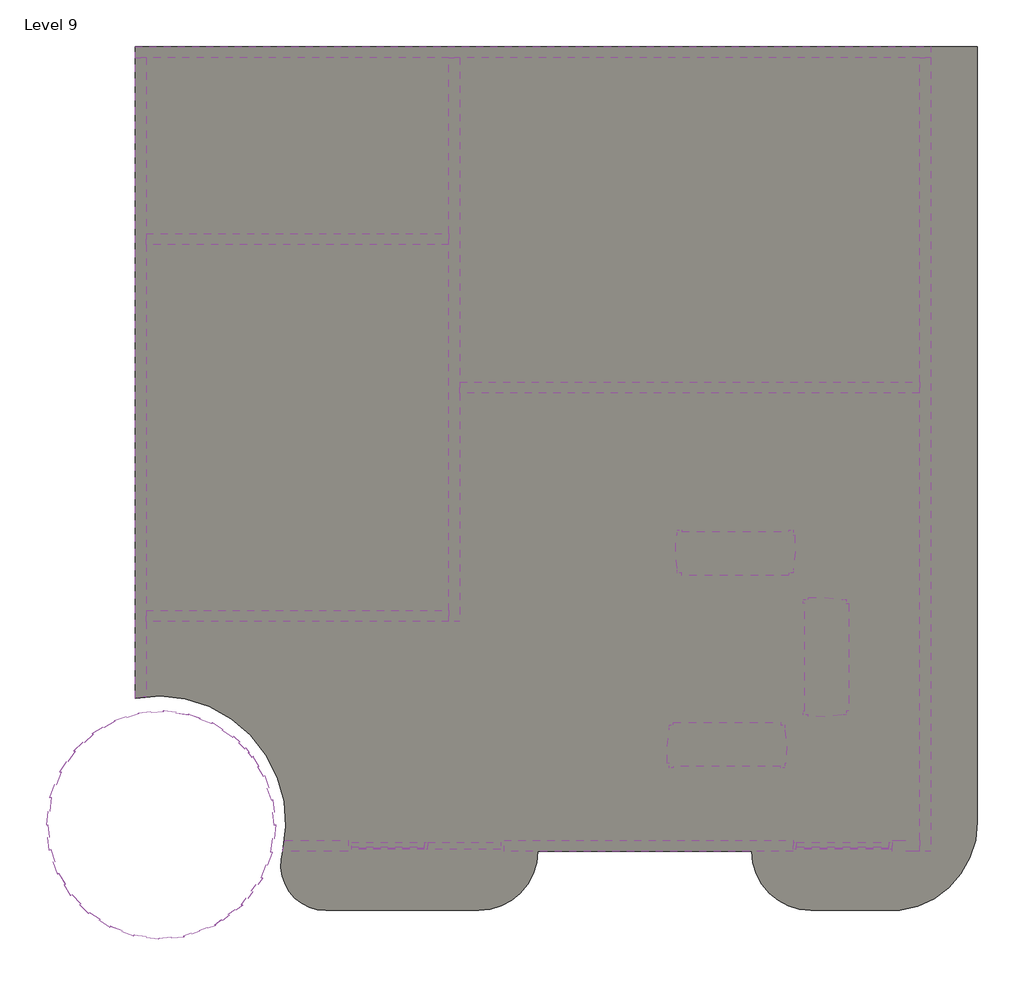
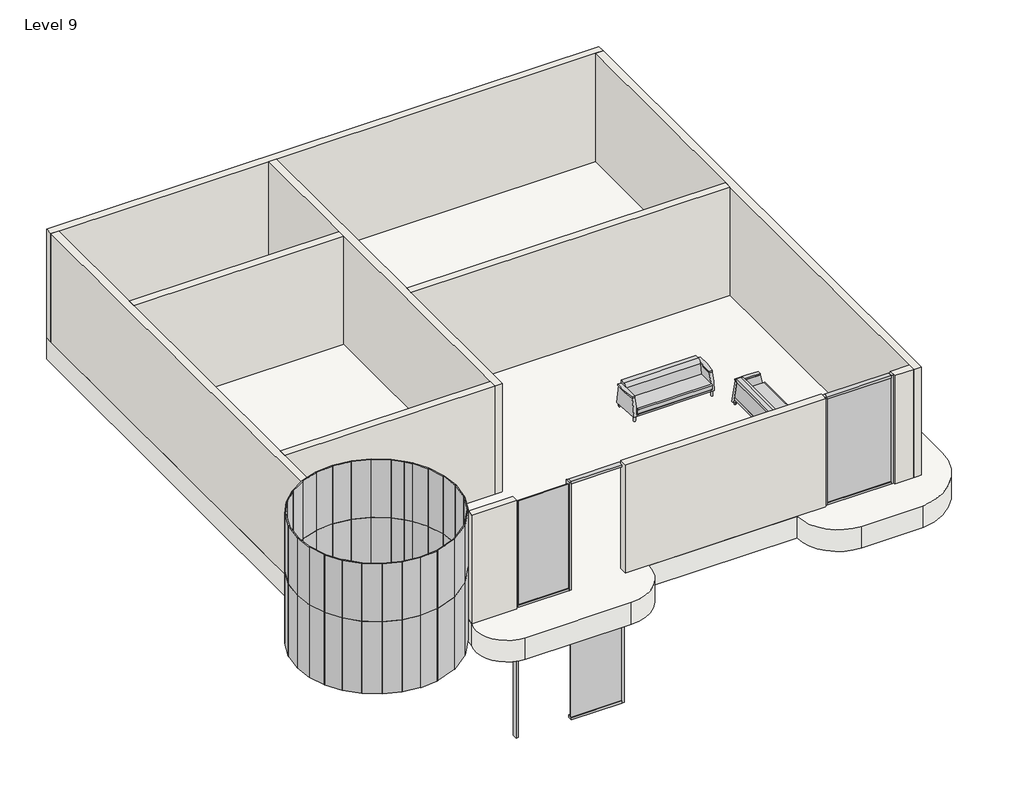
# One storey, incomplete: 59 plates, 11 members, 10 walls, 3 furniture elements, 1 slab.
"""IFC4 building model written with IfcOpenShell, lengths in millimetres."""

from ifc_helpers import new_model, si_unit, point, frame, frame_2d, origin, place, context, project, spatial, polyline, circle_curve, trimmed, segment, composite_curve, outline, extrude, faceted_brep, transform, mapped, element, save
from ifc_brep_helpers import plane_surface, revolved_surface, advanced_brep
from components import furniture_aff9b2fb, member_eaba9652, member_3f395ae9, member_0c868e12, member_7bc42366, system_panel_glazed_f1c144f9, system_panel_glazed_8ed2b2ee, system_panel_glazed_c7815b78, system_panel_glazed_220ba5f3, system_panel_glazed_11fb153e, system_panel_glazed_2f540b85, system_panel_glazed_4848e608, system_panel_glazed_8b35a0ff, system_panel_glazed_87282c25, system_panel_glazed_6d1bb68c, system_panel_glazed_cb3ffd69, system_panel_glazed_404d015f, system_panel_glazed_7b556abe, system_panel_glazed_370bf902

model = new_model("IFC4")

# Units and contexts
model_context = context("Model", 3, world=origin())
ifc_project = project(units=[si_unit("LENGTHUNIT", "METRE", prefix="MILLI")], contexts=[model_context])

# Site, building, storey
site = spatial("IfcSite", under=ifc_project)
building = spatial("IfcBuilding", under=site)
storey = spatial("IfcBuildingStorey", under=building, Name="Level 9", Elevation=24384.0)

# Furniture
placement = place(None, origin())
furniture_shape = furniture_aff9b2fb(model_context)
element("IfcFurniture", 1, ObjectType="Sofa-Pensi : 84\"", at=placement, inside=storey, context=model_context, shape_type="MappedRepresentation", body=[
    mapped(furniture_shape, transform((-2244.8524991, 3650.1964615, 25603.2), x_axis=(1.0, 0.0, 0.0), y_axis=(0.0, 1.0, 0.0), z_axis=(0.0, 0.0, 1.0))),
])
element("IfcFurniture", 2, ObjectType="Sofa-Pensi : 84\"", at=placement, inside=storey, context=model_context, shape_type="MappedRepresentation", body=[
    mapped(furniture_shape, transform((-12.736413, 1720.492712, 25603.2), x_axis=(0.0, 1.0, 0.0), y_axis=(-1.0, 0.0, 0.0), z_axis=(0.0, 0.0, 1.0))),
])
element("IfcFurniture", 3, ObjectType="Sofa-Pensi : 84\"", at=placement, inside=storey, context=model_context, shape_type="MappedRepresentation", body=[
    mapped(furniture_shape, transform((-1840.0399991, 648.4161336, 25603.2), x_axis=(-1.0, 0.0, 0.0), y_axis=(0.0, -1.0, 0.0), z_axis=(0.0, 0.0, 1.0))),
])

# Members
member_shape = member_eaba9652(model_context)
element("IfcMember", 4, ObjectType="Rectangular Mullion : 2.5\" x 5\" rectangular", at=placement, inside=storey, context=model_context, shape_type="MappedRepresentation", body=[
    mapped(member_shape, transform((-7672.5789001, -1482.8937024, 25603.2), x_axis=(-1.0, 0.0, 0.0), y_axis=(0.0, 1.0, 0.0), z_axis=(0.0, 0.0, -1.0))),
])
member_2_shape = member_3f395ae9(model_context)
element("IfcMember", 5, ObjectType="Rectangular Mullion : 2.5\" x 5\" rectangular", at=placement, inside=storey, context=model_context, shape_type="MappedRepresentation", body=[
    mapped(member_2_shape, transform((-9111.7115512, -1482.8937024, 21945.6), x_axis=(-1.0, 0.0, 0.0), y_axis=(0.0, 1.0, 0.0), z_axis=(0.0, 0.0, -1.0))),
])
element("IfcMember", 6, ObjectType="Rectangular Mullion : 2.5\" x 5\" rectangular", at=placement, inside=storey, context=model_context, shape_type="MappedRepresentation", body=[
    mapped(member_2_shape, transform((-899.4462491, -1482.8937024, 25603.2), x_axis=(-1.0, 0.0, 0.0), y_axis=(0.0, 1.0, 0.0), z_axis=(0.0, 0.0, -1.0))),
])
element("IfcMember", 7, ObjectType="Rectangular Mullion : 2.5\" x 5\" rectangular", at=placement, inside=storey, context=model_context, shape_type="MappedRepresentation", body=[
    mapped(member_2_shape, transform((-6233.4462491, -1482.8937024, 24993.6), x_axis=(1.0, 0.0, 0.0), y_axis=(0.0, 1.0, 0.0), z_axis=(0.0, 0.0, 1.0))),
])
element("IfcMember", 8, ObjectType="Rectangular Mullion : 2.5\" x 5\" rectangular", at=placement, inside=storey, context=model_context, shape_type="MappedRepresentation", body=[
    mapped(member_2_shape, transform((929.3537509, -1482.8937024, 28651.2), x_axis=(1.0, 0.0, 0.0), y_axis=(0.0, 1.0, 0.0), z_axis=(0.0, 0.0, 1.0))),
])
member_3_shape = member_0c868e12(model_context)
element("IfcMember", 9, ObjectType="Rectangular Mullion : 2.5\" x 5\" rectangular", at=placement, inside=storey, context=model_context, shape_type="MappedRepresentation", body=[
    mapped(member_3_shape, transform((-9048.2115512, -1482.8937024, 24993.6), x_axis=(0.0, 0.0, 1.0), y_axis=(0.0, 1.0, 0.0), z_axis=(-1.0, 0.0, 0.0))),
])
element("IfcMember", 10, ObjectType="Rectangular Mullion : 2.5\" x 5\" rectangular", at=placement, inside=storey, context=model_context, shape_type="MappedRepresentation", body=[
    mapped(member_3_shape, transform((-7640.8289001, -1482.8937024, 28651.2), x_axis=(0.0, 0.0, 1.0), y_axis=(0.0, 1.0, 0.0), z_axis=(-1.0, 0.0, 0.0))),
])
element("IfcMember", 11, ObjectType="Rectangular Mullion : 2.5\" x 5\" rectangular", at=placement, inside=storey, context=model_context, shape_type="MappedRepresentation", body=[
    mapped(member_3_shape, transform((-6296.9462491, -1482.8937024, 21945.6), x_axis=(0.0, 0.0, -1.0), y_axis=(0.0, 1.0, 0.0), z_axis=(1.0, 0.0, 0.0))),
])
element("IfcMember", 12, ObjectType="Rectangular Mullion : 2.5\" x 5\" rectangular", at=placement, inside=storey, context=model_context, shape_type="MappedRepresentation", body=[
    mapped(member_3_shape, transform((-7704.3289001, -1482.8937024, 25603.2), x_axis=(0.0, 0.0, -1.0), y_axis=(0.0, 1.0, 0.0), z_axis=(1.0, 0.0, 0.0))),
])
member_4_shape = member_7bc42366(model_context)
element("IfcMember", 13, ObjectType="Rectangular Mullion : 2.5\" x 5\" rectangular", at=placement, inside=storey, context=model_context, shape_type="MappedRepresentation", body=[
    mapped(member_4_shape, transform((-835.9462491, -1482.8937024, 28651.2), x_axis=(0.0, 0.0, 1.0), y_axis=(0.0, 1.0, 0.0), z_axis=(-1.0, 0.0, 0.0))),
])
element("IfcMember", 14, ObjectType="Rectangular Mullion : 2.5\" x 5\" rectangular", at=placement, inside=storey, context=model_context, shape_type="MappedRepresentation", body=[
    mapped(member_4_shape, transform((865.8537509, -1482.8937024, 25603.2), x_axis=(0.0, 0.0, -1.0), y_axis=(0.0, 1.0, 0.0), z_axis=(1.0, 0.0, 0.0))),
])

# Plates
system_panel_glazed_shape = system_panel_glazed_f1c144f9(model_context)
element("IfcPlate", 15, ObjectType="System Panel : Glazed", at=placement, inside=storey, context=model_context, shape_type="MappedRepresentation", body=[
    mapped(system_panel_glazed_shape, transform((-14541.9245022, -346.5978939, 25603.2), x_axis=(-0.3551689475306269, -0.9348021281051873, 0.0), y_axis=(0.9348021281051873, -0.3551689475306269, 0.0), z_axis=(0.0, 0.0, 1.0))),
])
element("IfcPlate", 16, ObjectType="System Panel : Glazed", at=placement, inside=storey, context=model_context, shape_type="MappedRepresentation", body=[
    mapped(system_panel_glazed_shape, transform((-10582.1178502, -1851.0877948, 25603.2), x_axis=(0.35516894753064066, 0.934802128105182, 0.0), y_axis=(-0.934802128105182, 0.35516894753064066, 0.0), z_axis=(0.0, 0.0, 1.0))),
])
element("IfcPlate", 17, ObjectType="System Panel : Glazed", at=placement, inside=storey, context=model_context, shape_type="MappedRepresentation", body=[
    mapped(system_panel_glazed_shape, transform((-10459.5232171, -1354.5613954, 25603.2), x_axis=(0.12073632210407237, 0.9926846128175765, 0.0), y_axis=(-0.9926846128175765, 0.12073632210407237, 0.0), z_axis=(0.0, 0.0, 1.0))),
])
element("IfcPlate", 18, ObjectType="System Panel : Glazed", at=placement, inside=storey, context=model_context, shape_type="MappedRepresentation", body=[
    mapped(system_panel_glazed_shape, transform((-14664.5191354, -843.1242933, 25603.2), x_axis=(-0.12073632210406239, -0.9926846128175777, 0.0), y_axis=(0.9926846128175777, -0.12073632210406239, 0.0), z_axis=(0.0, 0.0, 1.0))),
])
system_panel_glazed_2_shape = system_panel_glazed_8ed2b2ee(model_context)
element("IfcPlate", 19, ObjectType="System Panel : Glazed", at=placement, inside=storey, context=model_context, shape_type="MappedRepresentation", body=[
    mapped(system_panel_glazed_2_shape, transform((-11841.3777431, -3082.3793017, 25603.2), x_axis=(0.9398911711666007, 0.3414741371803665, 0.0), y_axis=(-0.3414741371803665, 0.9398911711666007, 0.0), z_axis=(0.0, 0.0, 1.0))),
])
element("IfcPlate", 20, ObjectType="System Panel : Glazed", at=placement, inside=storey, context=model_context, shape_type="MappedRepresentation", body=[
    mapped(system_panel_glazed_2_shape, transform((-10858.9635423, -2345.1728692, 25603.2), x_axis=(0.5905687200141164, 0.8069873524045393, 0.0), y_axis=(-0.8069873524045393, 0.5905687200141164, 0.0), z_axis=(0.0, 0.0, 1.0))),
])
element("IfcPlate", 21, ObjectType="System Panel : Glazed", at=placement, inside=storey, context=model_context, shape_type="MappedRepresentation", body=[
    mapped(system_panel_glazed_2_shape, transform((-11295.3522982, -2786.8279712, 25603.2), x_axis=(0.7998453025525061, 0.6002062078858317, 0.0), y_axis=(-0.6002062078858317, 0.7998453025525061, 0.0), z_axis=(0.0, 0.0, 1.0))),
])
system_panel_glazed_3_shape = system_panel_glazed_c7815b78(model_context)
element("IfcPlate", 22, ObjectType="System Panel : Glazed", at=placement, inside=storey, context=model_context, shape_type="MappedRepresentation", body=[
    mapped(system_panel_glazed_3_shape, transform((-10454.4737362, -864.5204039, 25603.2), x_axis=(-0.11050163420416614, 0.993875942378227, 0.0), y_axis=(-0.993875942378227, -0.11050163420416614, 0.0), z_axis=(0.0, 0.0, 1.0))),
])
element("IfcPlate", 23, ObjectType="System Panel : Glazed", at=placement, inside=storey, context=model_context, shape_type="MappedRepresentation", body=[
    mapped(system_panel_glazed_3_shape, transform((-14669.5686163, -1333.1652848, 25603.2), x_axis=(0.11050163420415136, -0.9938759423782286, 0.0), y_axis=(0.9938759423782286, 0.11050163420415136, 0.0), z_axis=(0.0, 0.0, 1.0))),
])
element("IfcPlate", 24, ObjectType="System Panel : Glazed", at=placement, inside=storey, context=model_context, shape_type="MappedRepresentation", body=[
    mapped(system_panel_glazed_3_shape, transform((-11410.1424167, 681.5611944, 25603.2), x_axis=(-0.8396018558176894, 0.5432022861766066, 0.0), y_axis=(-0.5432022861766066, -0.8396018558176894, 0.0), z_axis=(0.0, 0.0, 1.0))),
])
element("IfcPlate", 25, ObjectType="System Panel : Glazed", at=placement, inside=storey, context=model_context, shape_type="MappedRepresentation", body=[
    mapped(system_panel_glazed_3_shape, transform((-13212.0893695, 919.590846, 25603.2), x_axis=(-0.9518517343814786, -0.3065587639506839, 0.0), y_axis=(0.3065587639506839, -0.9518517343814786, 0.0), z_axis=(0.0, 0.0, 1.0))),
])
element("IfcPlate", 26, ObjectType="System Panel : Glazed", at=placement, inside=storey, context=model_context, shape_type="MappedRepresentation", body=[
    mapped(system_panel_glazed_3_shape, transform((-12839.7224363, -3201.1142893, 25603.2), x_axis=(0.9913878918151698, -0.1309581916577702, 0.0), y_axis=(0.1309581916577702, 0.9913878918151698, 0.0), z_axis=(0.0, 0.0, 1.0))),
])
element("IfcPlate", 27, ObjectType="System Panel : Glazed", at=placement, inside=storey, context=model_context, shape_type="MappedRepresentation", body=[
    mapped(system_panel_glazed_3_shape, transform((-14365.783041, -2213.7896382, 25603.2), x_axis=(0.5257859322352114, -0.8506169252157811, 0.0), y_axis=(0.8506169252157811, 0.5257859322352114, 0.0), z_axis=(0.0, 0.0, 1.0))),
])
element("IfcPlate", 28, ObjectType="System Panel : Glazed", at=placement, inside=storey, context=model_context, shape_type="MappedRepresentation", body=[
    mapped(system_panel_glazed_3_shape, transform((-13713.8999358, -2879.2468831, 25603.2), x_axis=(0.8396018558176805, -0.5432022861766201, 0.0), y_axis=(0.5432022861766201, 0.8396018558176805, 0.0), z_axis=(0.0, 0.0, 1.0))),
])
element("IfcPlate", 29, ObjectType="System Panel : Glazed", at=placement, inside=storey, context=model_context, shape_type="MappedRepresentation", body=[
    mapped(system_panel_glazed_3_shape, transform((-14014.4059364, 446.2272921, 25603.2), x_axis=(-0.7286232370002992, -0.6849147235263715, 0.0), y_axis=(0.6849147235263715, -0.7286232370002992, 0.0), z_axis=(0.0, 0.0, 1.0))),
])
element("IfcPlate", 30, ObjectType="System Panel : Glazed", at=placement, inside=storey, context=model_context, shape_type="MappedRepresentation", body=[
    mapped(system_panel_glazed_3_shape, transform((-12284.3199161, 1003.4286006, 25603.2), x_axis=(-0.9913878918151723, 0.13095819165775144, 0.0), y_axis=(-0.13095819165775144, -0.9913878918151723, 0.0), z_axis=(0.0, 0.0, 1.0))),
])
element("IfcPlate", 31, ObjectType="System Panel : Glazed", at=placement, inside=storey, context=model_context, shape_type="MappedRepresentation", body=[
    mapped(system_panel_glazed_3_shape, transform((-12752.8652893, 1013.0855973, 25603.2), x_axis=(-0.9959419324521102, -0.08999815100076568, 0.0), y_axis=(0.08999815100076568, -0.9959419324521102, 0.0), z_axis=(0.0, 0.0, 1.0))),
])
element("IfcPlate", 32, ObjectType="System Panel : Glazed", at=placement, inside=storey, context=model_context, shape_type="MappedRepresentation", body=[
    mapped(system_panel_glazed_3_shape, transform((-11829.3381514, 891.0915272, 25603.2), x_axis=(-0.9384120429483949, 0.3455182160891376, 0.0), y_axis=(-0.3455182160891376, -0.9384120429483949, 0.0), z_axis=(0.0, 0.0, 1.0))),
])
element("IfcPlate", 33, ObjectType="System Panel : Glazed", at=placement, inside=storey, context=model_context, shape_type="MappedRepresentation", body=[
    mapped(system_panel_glazed_3_shape, transform((-10557.4115054, -407.3204039, 25603.2), x_axis=(-0.3261077326604367, 0.9453326116764772, 0.0), y_axis=(-0.9453326116764772, -0.3261077326604367, 0.0), z_axis=(0.0, 0.0, 1.0))),
])
element("IfcPlate", 34, ObjectType="System Panel : Glazed", at=placement, inside=storey, context=model_context, shape_type="MappedRepresentation", body=[
    mapped(system_panel_glazed_3_shape, transform((-12371.1770631, -3210.771286, 25603.2), x_axis=(0.9959419324521115, 0.08999815100075001, 0.0), y_axis=(-0.08999815100075001, 0.9959419324521115, 0.0), z_axis=(0.0, 0.0, 1.0))),
])
element("IfcPlate", 35, ObjectType="System Panel : Glazed", at=placement, inside=storey, context=model_context, shape_type="MappedRepresentation", body=[
    mapped(system_panel_glazed_3_shape, transform((-13294.7042011, -3088.7772159, 25603.2), x_axis=(0.9384120429483891, -0.34551821608915334, 0.0), y_axis=(0.34551821608915334, 0.9384120429483891, 0.0), z_axis=(0.0, 0.0, 1.0))),
])
element("IfcPlate", 36, ObjectType="System Panel : Glazed", at=placement, inside=storey, context=model_context, shape_type="MappedRepresentation", body=[
    mapped(system_panel_glazed_3_shape, transform((-14076.8350959, -2582.7572647, 25603.2), x_axis=(0.6997834615185511, -0.7143550286692988, 0.0), y_axis=(0.7143550286692988, 0.6997834615185511, 0.0), z_axis=(0.0, 0.0, 1.0))),
])
element("IfcPlate", 37, ObjectType="System Panel : Glazed", at=placement, inside=storey, context=model_context, shape_type="MappedRepresentation", body=[
    mapped(system_panel_glazed_3_shape, transform((-14566.6308471, -1790.3652848, 25603.2), x_axis=(0.32610773266042153, -0.9453326116764824, 0.0), y_axis=(0.9453326116764824, 0.32610773266042153, 0.0), z_axis=(0.0, 0.0, 1.0))),
])
element("IfcPlate", 38, ObjectType="System Panel : Glazed", at=placement, inside=storey, context=model_context, shape_type="MappedRepresentation", body=[
    mapped(system_panel_glazed_3_shape, transform((-14318.3113206, 89.4787227, 25603.2), x_axis=(-0.5603879632167612, -0.8282302401396425, 0.0), y_axis=(0.8282302401396425, -0.5603879632167612, 0.0), z_axis=(0.0, 0.0, 1.0))),
])
element("IfcPlate", 39, ObjectType="System Panel : Glazed", at=placement, inside=storey, context=model_context, shape_type="MappedRepresentation", body=[
    mapped(system_panel_glazed_3_shape, transform((-13639.5625299, 727.5108588, 25603.2), x_axis=(-0.8612707706620224, -0.5081462974412448, 0.0), y_axis=(0.5081462974412448, -0.8612707706620224, 0.0), z_axis=(0.0, 0.0, 1.0))),
])
system_panel_glazed_4_shape = system_panel_glazed_220ba5f3(model_context)
element("IfcPlate", 40, ObjectType="System Panel : Glazed", at=placement, inside=storey, context=model_context, shape_type="MappedRepresentation", body=[
    mapped(system_panel_glazed_4_shape, transform((-10742.3305673, -4.7597883, 25603.2), x_axis=(-0.5152811917631037, 0.8570211744263939, 0.0), y_axis=(-0.8570211744263939, -0.5152811917631037, 0.0), z_axis=(0.0, 0.0, 1.0))),
])
system_panel_glazed_5_shape = system_panel_glazed_11fb153e(model_context)
element("IfcPlate", 41, ObjectType="System Panel : Glazed", at=placement, inside=storey, context=model_context, shape_type="MappedRepresentation", body=[
    mapped(system_panel_glazed_5_shape, transform((-11098.0043985, 445.2241463, 25603.2), x_axis=(-0.7256671855033587, 0.6880458821064435, 0.0), y_axis=(-0.6880458821064435, -0.7256671855033587, 0.0), z_axis=(0.0, 0.0, 1.0))),
])
system_panel_glazed_6_shape = system_panel_glazed_2f540b85(model_context)
element("IfcPlate", 42, ObjectType="System Panel : Glazed", at=placement, inside=storey, context=model_context, shape_type="MappedRepresentation", body=[
    mapped(system_panel_glazed_6_shape, transform((-10917.0903061, 255.9395759, 25603.2), x_axis=(-0.6357445726375757, 0.7718995001694627, 0.0), y_axis=(-0.7718995001694627, -0.6357445726375757, 0.0), z_axis=(0.0, 0.0, 1.0))),
])
system_panel_glazed_7_shape = system_panel_glazed_4848e608(model_context)
element("IfcPlate", 43, ObjectType="System Panel : Glazed", at=placement, inside=storey, context=model_context, shape_type="MappedRepresentation", body=[
    mapped(system_panel_glazed_7_shape, transform((-14669.5686163, -1333.1652848, 27635.2), x_axis=(0.11050163420415136, -0.9938759423782286, 0.0), y_axis=(0.9938759423782286, 0.11050163420415136, 0.0), z_axis=(0.0, 0.0, 1.0))),
])
element("IfcPlate", 44, ObjectType="System Panel : Glazed", at=placement, inside=storey, context=model_context, shape_type="MappedRepresentation", body=[
    mapped(system_panel_glazed_7_shape, transform((-14365.783041, -2213.7896382, 27635.2), x_axis=(0.5257859322352114, -0.8506169252157811, 0.0), y_axis=(0.8506169252157811, 0.5257859322352114, 0.0), z_axis=(0.0, 0.0, 1.0))),
])
element("IfcPlate", 45, ObjectType="System Panel : Glazed", at=placement, inside=storey, context=model_context, shape_type="MappedRepresentation", body=[
    mapped(system_panel_glazed_7_shape, transform((-13713.8999358, -2879.2468831, 27635.2), x_axis=(0.8396018558176805, -0.5432022861766201, 0.0), y_axis=(0.5432022861766201, 0.8396018558176805, 0.0), z_axis=(0.0, 0.0, 1.0))),
])
element("IfcPlate", 46, ObjectType="System Panel : Glazed", at=placement, inside=storey, context=model_context, shape_type="MappedRepresentation", body=[
    mapped(system_panel_glazed_7_shape, transform((-12839.7224363, -3201.1142893, 27635.2), x_axis=(0.9913878918151698, -0.13095819165777017, 0.0), y_axis=(0.13095819165777017, 0.9913878918151698, 0.0), z_axis=(0.0, 0.0, 1.0))),
])
element("IfcPlate", 47, ObjectType="System Panel : Glazed", at=placement, inside=storey, context=model_context, shape_type="MappedRepresentation", body=[
    mapped(system_panel_glazed_7_shape, transform((-12371.1770631, -3210.771286, 27635.2), x_axis=(0.9959419324521115, 0.08999815100075001, 0.0), y_axis=(-0.08999815100075001, 0.9959419324521115, 0.0), z_axis=(0.0, 0.0, 1.0))),
])
element("IfcPlate", 48, ObjectType="System Panel : Glazed", at=placement, inside=storey, context=model_context, shape_type="MappedRepresentation", body=[
    mapped(system_panel_glazed_7_shape, transform((-13294.7042011, -3088.7772159, 27635.2), x_axis=(0.9384120429483891, -0.34551821608915334, 0.0), y_axis=(0.34551821608915334, 0.9384120429483891, 0.0), z_axis=(0.0, 0.0, 1.0))),
])
element("IfcPlate", 49, ObjectType="System Panel : Glazed", at=placement, inside=storey, context=model_context, shape_type="MappedRepresentation", body=[
    mapped(system_panel_glazed_7_shape, transform((-14076.8350959, -2582.7572647, 27635.2), x_axis=(0.6997834615185511, -0.7143550286692988, 0.0), y_axis=(0.7143550286692988, 0.6997834615185511, 0.0), z_axis=(0.0, 0.0, 1.0))),
])
element("IfcPlate", 50, ObjectType="System Panel : Glazed", at=placement, inside=storey, context=model_context, shape_type="MappedRepresentation", body=[
    mapped(system_panel_glazed_7_shape, transform((-14566.6308471, -1790.3652848, 27635.2), x_axis=(0.32610773266042153, -0.9453326116764824, 0.0), y_axis=(0.9453326116764824, 0.32610773266042153, 0.0), z_axis=(0.0, 0.0, 1.0))),
])
element("IfcPlate", 51, ObjectType="System Panel : Glazed", at=placement, inside=storey, context=model_context, shape_type="MappedRepresentation", body=[
    mapped(system_panel_glazed_7_shape, transform((-10454.4737362, -864.5204039, 27635.2), x_axis=(-0.11050163420416614, 0.993875942378227, 0.0), y_axis=(-0.993875942378227, -0.11050163420416614, 0.0), z_axis=(0.0, 0.0, 1.0))),
])
element("IfcPlate", 52, ObjectType="System Panel : Glazed", at=placement, inside=storey, context=model_context, shape_type="MappedRepresentation", body=[
    mapped(system_panel_glazed_7_shape, transform((-10557.4115054, -407.3204039, 27635.2), x_axis=(-0.3261077326604368, 0.9453326116764772, 0.0), y_axis=(-0.9453326116764772, -0.3261077326604368, 0.0), z_axis=(0.0, 0.0, 1.0))),
])
element("IfcPlate", 53, ObjectType="System Panel : Glazed", at=placement, inside=storey, context=model_context, shape_type="MappedRepresentation", body=[
    mapped(system_panel_glazed_7_shape, transform((-11410.1424167, 681.5611944, 27635.2), x_axis=(-0.8396018558176894, 0.5432022861766066, 0.0), y_axis=(-0.5432022861766066, -0.8396018558176894, 0.0), z_axis=(0.0, 0.0, 1.0))),
])
element("IfcPlate", 54, ObjectType="System Panel : Glazed", at=placement, inside=storey, context=model_context, shape_type="MappedRepresentation", body=[
    mapped(system_panel_glazed_7_shape, transform((-11829.3381514, 891.0915272, 27635.2), x_axis=(-0.9384120429483949, 0.3455182160891376, 0.0), y_axis=(-0.3455182160891376, -0.9384120429483949, 0.0), z_axis=(0.0, 0.0, 1.0))),
])
element("IfcPlate", 55, ObjectType="System Panel : Glazed", at=placement, inside=storey, context=model_context, shape_type="MappedRepresentation", body=[
    mapped(system_panel_glazed_7_shape, transform((-12284.3199161, 1003.4286006, 27635.2), x_axis=(-0.9913878918151723, 0.1309581916577514, 0.0), y_axis=(-0.1309581916577514, -0.9913878918151723, 0.0), z_axis=(0.0, 0.0, 1.0))),
])
element("IfcPlate", 56, ObjectType="System Panel : Glazed", at=placement, inside=storey, context=model_context, shape_type="MappedRepresentation", body=[
    mapped(system_panel_glazed_7_shape, transform((-12752.8652893, 1013.0855973, 27635.2), x_axis=(-0.9959419324521102, -0.08999815100076568, 0.0), y_axis=(0.08999815100076568, -0.9959419324521102, 0.0), z_axis=(0.0, 0.0, 1.0))),
])
element("IfcPlate", 57, ObjectType="System Panel : Glazed", at=placement, inside=storey, context=model_context, shape_type="MappedRepresentation", body=[
    mapped(system_panel_glazed_7_shape, transform((-13212.0893695, 919.590846, 27635.2), x_axis=(-0.9518517343814786, -0.3065587639506839, 0.0), y_axis=(0.3065587639506839, -0.9518517343814786, 0.0), z_axis=(0.0, 0.0, 1.0))),
])
element("IfcPlate", 58, ObjectType="System Panel : Glazed", at=placement, inside=storey, context=model_context, shape_type="MappedRepresentation", body=[
    mapped(system_panel_glazed_7_shape, transform((-13639.5625299, 727.5108588, 27635.2), x_axis=(-0.8612707706620223, -0.508146297441245, 0.0), y_axis=(0.508146297441245, -0.8612707706620223, 0.0), z_axis=(0.0, 0.0, 1.0))),
])
element("IfcPlate", 59, ObjectType="System Panel : Glazed", at=placement, inside=storey, context=model_context, shape_type="MappedRepresentation", body=[
    mapped(system_panel_glazed_7_shape, transform((-14014.4059364, 446.2272921, 27635.2), x_axis=(-0.7286232370002992, -0.6849147235263715, 0.0), y_axis=(0.6849147235263715, -0.7286232370002992, 0.0), z_axis=(0.0, 0.0, 1.0))),
])
element("IfcPlate", 60, ObjectType="System Panel : Glazed", at=placement, inside=storey, context=model_context, shape_type="MappedRepresentation", body=[
    mapped(system_panel_glazed_7_shape, transform((-14318.3113206, 89.4787227, 27635.2), x_axis=(-0.5603879632167612, -0.8282302401396425, 0.0), y_axis=(0.8282302401396425, -0.5603879632167612, 0.0), z_axis=(0.0, 0.0, 1.0))),
])
system_panel_glazed_8_shape = system_panel_glazed_8b35a0ff(model_context)
element("IfcPlate", 61, ObjectType="System Panel : Glazed", at=placement, inside=storey, context=model_context, shape_type="MappedRepresentation", body=[
    mapped(system_panel_glazed_8_shape, transform((-10742.3305673, -4.7597883, 27635.2), x_axis=(-0.5152811917631037, 0.8570211744263939, 0.0), y_axis=(-0.8570211744263939, -0.5152811917631037, 0.0), z_axis=(0.0, 0.0, 1.0))),
])
system_panel_glazed_9_shape = system_panel_glazed_87282c25(model_context)
element("IfcPlate", 62, ObjectType="System Panel : Glazed", at=placement, inside=storey, context=model_context, shape_type="MappedRepresentation", body=[
    mapped(system_panel_glazed_9_shape, transform((-10917.0903061, 255.9395759, 27635.2), x_axis=(-0.6357445726375757, 0.7718995001694627, 0.0), y_axis=(-0.7718995001694627, -0.6357445726375757, 0.0), z_axis=(0.0, 0.0, 1.0))),
])
system_panel_glazed_10_shape = system_panel_glazed_6d1bb68c(model_context)
element("IfcPlate", 63, ObjectType="System Panel : Glazed", at=placement, inside=storey, context=model_context, shape_type="MappedRepresentation", body=[
    mapped(system_panel_glazed_10_shape, transform((-11098.0043985, 445.2241463, 27635.2), x_axis=(-0.7256671855033587, 0.6880458821064435, 0.0), y_axis=(-0.6880458821064435, -0.7256671855033587, 0.0), z_axis=(0.0, 0.0, 1.0))),
])
system_panel_glazed_11_shape = system_panel_glazed_cb3ffd69(model_context)
element("IfcPlate", 64, ObjectType="System Panel : Glazed", at=placement, inside=storey, context=model_context, shape_type="MappedRepresentation", body=[
    mapped(system_panel_glazed_11_shape, transform((-10582.1178502, -1851.0877948, 27635.2), x_axis=(0.35516894753064066, 0.934802128105182, 0.0), y_axis=(-0.934802128105182, 0.35516894753064066, 0.0), z_axis=(0.0, 0.0, 1.0))),
])
element("IfcPlate", 65, ObjectType="System Panel : Glazed", at=placement, inside=storey, context=model_context, shape_type="MappedRepresentation", body=[
    mapped(system_panel_glazed_11_shape, transform((-10459.5232171, -1354.5613954, 27635.2), x_axis=(0.1207363221040724, 0.9926846128175765, 0.0), y_axis=(-0.9926846128175765, 0.1207363221040724, 0.0), z_axis=(0.0, 0.0, 1.0))),
])
element("IfcPlate", 66, ObjectType="System Panel : Glazed", at=placement, inside=storey, context=model_context, shape_type="MappedRepresentation", body=[
    mapped(system_panel_glazed_11_shape, transform((-14541.9245022, -346.5978939, 27635.2), x_axis=(-0.3551689475306269, -0.9348021281051873, 0.0), y_axis=(0.9348021281051873, -0.3551689475306269, 0.0), z_axis=(0.0, 0.0, 1.0))),
])
element("IfcPlate", 67, ObjectType="System Panel : Glazed", at=placement, inside=storey, context=model_context, shape_type="MappedRepresentation", body=[
    mapped(system_panel_glazed_11_shape, transform((-14664.5191354, -843.1242933, 27635.2), x_axis=(-0.1207363221040624, -0.9926846128175777, 0.0), y_axis=(0.9926846128175777, -0.1207363221040624, 0.0), z_axis=(0.0, 0.0, 1.0))),
])
system_panel_glazed_12_shape = system_panel_glazed_404d015f(model_context)
element("IfcPlate", 68, ObjectType="System Panel : Glazed", at=placement, inside=storey, context=model_context, shape_type="MappedRepresentation", body=[
    mapped(system_panel_glazed_12_shape, transform((-11841.3777431, -3082.3793017, 27635.2), x_axis=(0.9398911711666007, 0.3414741371803665, 0.0), y_axis=(-0.3414741371803665, 0.9398911711666007, 0.0), z_axis=(0.0, 0.0, 1.0))),
])
element("IfcPlate", 69, ObjectType="System Panel : Glazed", at=placement, inside=storey, context=model_context, shape_type="MappedRepresentation", body=[
    mapped(system_panel_glazed_12_shape, transform((-10858.9635423, -2345.1728692, 27635.2), x_axis=(0.5905687200141164, 0.8069873524045393, 0.0), y_axis=(-0.8069873524045393, 0.5905687200141164, 0.0), z_axis=(0.0, 0.0, 1.0))),
])
element("IfcPlate", 70, ObjectType="System Panel : Glazed", at=placement, inside=storey, context=model_context, shape_type="MappedRepresentation", body=[
    mapped(system_panel_glazed_12_shape, transform((-11295.3522982, -2786.8279712, 27635.2), x_axis=(0.7998453025525062, 0.6002062078858316, 0.0), y_axis=(-0.6002062078858316, 0.7998453025525062, 0.0), z_axis=(0.0, 0.0, 1.0))),
])
system_panel_glazed_13_shape = system_panel_glazed_7b556abe(model_context)
element("IfcPlate", 71, ObjectType="System Panel : Glazed", at=placement, inside=storey, context=model_context, shape_type="MappedRepresentation", body=[
    mapped(system_panel_glazed_13_shape, transform((-6968.8875746, -1482.8937024, 22009.1), x_axis=(-1.0, 0.0, 0.0), y_axis=(0.0, -1.0, 0.0), z_axis=(0.0, 0.0, 1.0))),
])
element("IfcPlate", 72, ObjectType="System Panel : Glazed", at=placement, inside=storey, context=model_context, shape_type="MappedRepresentation", body=[
    mapped(system_panel_glazed_13_shape, transform((-8376.2702257, -1482.8937024, 25666.7), x_axis=(-1.0, 0.0, 0.0), y_axis=(0.0, -1.0, 0.0), z_axis=(0.0, 0.0, 1.0))),
])
system_panel_glazed_14_shape = system_panel_glazed_370bf902(model_context)
element("IfcPlate", 73, ObjectType="System Panel : Glazed", at=placement, inside=storey, context=model_context, shape_type="MappedRepresentation", body=[
    mapped(system_panel_glazed_14_shape, transform((14.9537509, -1482.8937024, 25666.7), x_axis=(-1.0, 0.0, 0.0), y_axis=(0.0, -1.0, 0.0), z_axis=(0.0, 0.0, 1.0))),
])

# Slab
element("IfcSlab", 74, ObjectType="Generic - 2'", at=placement, inside=storey, context=model_context, shape_type="SweptSolid", body=[
    extrude(outline(composite_curve([segment(polyline([(2504.1537509, 13274.5062976), (2504.1537509, -1051.0937024)]), True, "CONTINUOUS"), segment(trimmed(circle_curve(frame_2d((865.9099456, -1051.0937024)), 1638.2438053), [point((2504.1537509, -1051.0937024))], [point((1069.0537509, -2676.6937024))], False, "CARTESIAN"), True, "CONTINUOUS"), segment(polyline([(1069.0537509, -2676.6937024), (-569.2462491, -2676.6937024)]), True, "CONTINUOUS"), segment(trimmed(circle_curve(frame_2d((-569.2462491, -1584.4937024)), 1092.2), [point((-569.2462491, -2676.6937024))], [point((-1661.4462491, -1584.4937024))], False, "CARTESIAN"), True, "CONTINUOUS"), segment(polyline([(-1661.4462491, -1584.4937024), (-5609.8647377, -1584.4937024)]), True, "CONTINUOUS"), segment(trimmed(circle_curve(frame_2d((-6702.0647377, -1584.4937024)), 1092.2), [point((-5609.8647377, -1584.4937024))], [point((-6702.0647377, -2676.6937024))], False, "CARTESIAN"), True, "CONTINUOUS"), segment(polyline([(-6702.0647377, -2676.6937024), (-9521.4647377, -2676.6937024)]), True, "CONTINUOUS"), segment(trimmed(circle_curve(frame_2d((-9521.4647377, -1843.8920375)), 832.801665), [point((-9521.4647377, -2676.6937024))], [point((-10312.8376694, -1584.4937024))], False, "CARTESIAN"), True, "CONTINUOUS"), segment(trimmed(circle_curve(frame_2d((-12612.6150686, -1075.1054509)), 2355.5153315), [point((-10312.8376694, -1584.4937024))], [point((-13040.6462491, 1241.1937063))], True, "CARTESIAN"), True, "CONTINUOUS"), segment(polyline([(-13040.6462491, 1241.1937063), (-13040.6462491, 13274.5062976), (2504.1537509, 13274.5062976)]), True, "CONTINUOUS")], self_intersect=False)), frame((0.0, 0.0, 24993.6), z_axis=(0.0, 0.0, 1.0), x_axis=(1.0, 0.0, 0.0)), (0.0, 0.0, 1.0), 609.6),
])

# Walls
element("IfcWall", 75, ObjectType="Generic - 8\"", at=placement, inside=storey, context=model_context, shape_type="Brep", body=[
    faceted_brep([(-13040.6462491, 13071.3062976, 25603.2), (-12837.4462491, 13071.3062976, 25603.2), (-7249.4462491, 13071.3062976, 25603.2), (-7046.2462491, 13071.3062976, 25603.2), (1437.3537509, 13071.3062976, 25603.2), (1640.5537509, 13071.3062976, 25603.2), (1640.5537509, 13071.3062976, 28651.2), (1437.3537509, 13071.3062976, 28651.2), (-7046.2462491, 13071.3062976, 28651.2), (-7249.4462491, 13071.3062976, 28651.2), (-12837.4462491, 13071.3062976, 28651.2), (-13040.6462491, 13071.3062976, 28651.2), (-13040.6462491, 13274.5062976, 25603.2), (-13040.6462491, 13274.5062976, 28651.2), (1640.5537509, 13274.5062976, 28651.2), (1640.5537509, 13274.5062976, 25603.2)], [[[0, 1, 2, 3, 4, 5, 6, 7, 8, 9, 10, 11]], [[12, 13, 14, 15]], [[5, 4, 3, 2, 1, 0, 12, 15]], [[11, 10, 9, 8, 7, 6, 14, 13]], [[6, 5, 15, 14]], [[0, 11, 13, 12]]]),
])
element("IfcWall", 76, ObjectType="Generic - 8\"", at=placement, inside=storey, context=model_context, shape_type="Brep", body=[
    faceted_brep([(1437.3537509, 13071.3062976, 25603.2), (1437.3537509, 7076.9062976, 25603.2), (1437.3537509, 6873.7062976, 25603.2), (1437.3537509, -1381.2937024, 25603.2), (1437.3537509, -1584.4937024, 25603.2), (1437.3537509, -1584.4937024, 28651.2), (1437.3537509, -1381.2937024, 28651.2), (1437.3537509, 6873.7062976, 28651.2), (1437.3537509, 7076.9062976, 28651.2), (1437.3537509, 13071.3062976, 28651.2), (1640.5537509, 13071.3062976, 25603.2), (1640.5537509, 13071.3062976, 28651.2), (1640.5537509, -1584.4937024, 28651.2), (1640.5537509, -1584.4937024, 25603.2)], [[[0, 1, 2, 3, 4, 5, 6, 7, 8, 9]], [[10, 11, 12, 13]], [[4, 3, 2, 1, 0, 10, 13]], [[9, 8, 7, 6, 5, 12, 11]], [[0, 9, 11, 10]], [[5, 4, 13, 12]]]),
])
element("IfcWall", 77, ObjectType="Generic - 8\"", at=placement, inside=storey, context=model_context, shape_type="AdvancedBrep", body=[
    advanced_brep(
    [(-13040.6462491, 13071.3062976, 25603.2), (-13040.6462491, 1241.1937063, 25603.2), (-13040.6462491, 1241.1937063, 28651.2), (-13040.6462491, 13071.3062976, 28651.2), (-12837.4462491, 13071.3062976, 25603.2), (-12837.4462491, 13071.3062976, 28651.2), (-12837.4462491, 9820.1062976, 28651.2), (-12837.4462491, 9616.9062976, 28651.2), (-12837.4462491, 2862.698962, 28651.2), (-12837.4462491, 2659.498962, 28651.2), (-12837.4462491, 1269.6553935, 28651.2), (-12837.4462491, 1269.6553935, 25603.2), (-12837.4462491, 2659.498962, 25603.2), (-12837.4462491, 2862.698962, 25603.2), (-12837.4462491, 9616.9062976, 25603.2), (-12837.4462491, 9820.1062976, 25603.2)],
    [
        (0, 1),
        (1, 2),
        (2, 3),
        (3, 0),
        (4, 5),
        (5, 6),
        (6, 7),
        (7, 8),
        (8, 9),
        (9, 10),
        (10, 11),
        (11, 12),
        (12, 13),
        (13, 14),
        (14, 15),
        (15, 4),
        (0, 4),
        (11, 1, circle_curve(frame((-12612.6150686, -1075.1054509, 25603.2), z_axis=(0.0, 0.0, 1.0), x_axis=(1.0, 0.0, 0.0)), 2355.5153315)),
        (2, 10, circle_curve(frame((-12612.6150686, -1075.1054509, 28651.2), z_axis=(0.0, 0.0, -1.0), x_axis=(1.0, 0.0, 0.0)), 2355.5153315)),
        (5, 3),
    ],
    [
        plane_surface(frame((-13040.6462491, 16068.5062976, 25603.2), z_axis=(-1.0, 0.0, 0.0), x_axis=(0.0, -1.0, 0.0))),
        plane_surface(frame((-12837.4462491, 16068.5062976, 25603.2), z_axis=(1.0, 0.0, 0.0), x_axis=(0.0, 1.0, 0.0))),
        plane_surface(frame((-13040.6462491, 13172.9062976, 25603.2), z_axis=(0.0, 0.0, -1.0), x_axis=(1.0, 0.0, 0.0))),
        plane_surface(frame((-13040.6462491, 1155.046339, 28651.2), z_axis=(0.0, 0.0, 1.0), x_axis=(1.0, 0.0, 0.0))),
        plane_surface(frame((-16139.4462491, 13071.3062976, 25603.2), z_axis=(0.0, 1.0, 0.0), x_axis=(1.0, 0.0, 0.0))),
        revolved_surface(polyline([(-10257.099737100001, -1075.1054509, 28651.2), (-10257.099737100001, -1075.1054509, 25603.2)]), (-12612.6150686, -1075.1054509, 25603.2), (0.0, 0.0, 1.0)),
    ],
    [
        (0, [[1, 2, 3, 4]]),
        (1, [[5, 6, 7, 8, 9, 10, 11, 12, 13, 14, 15, 16]]),
        (2, [[-1, 17, -16, -15, -14, -13, -12, 18]]),
        (3, [[-3, 19, -10, -9, -8, -7, -6, 20]]),
        (4, [[-4, -20, -5, -17]]),
        (5, [[-2, -18, -11, -19]]),
    ],
),
])
element("IfcWall", 78, ObjectType="Generic - 8\"", at=placement, inside=storey, context=model_context, shape_type="Brep", body=[
    faceted_brep([(-7249.4462491, 13071.3062976, 25603.2), (-7249.4462491, 9820.1062976, 25603.2), (-7249.4462491, 9616.9062976, 25603.2), (-7249.4462491, 2862.698962, 25603.2), (-7249.4462491, 2659.498962, 25603.2), (-7249.4462491, 2659.498962, 28651.2), (-7249.4462491, 2862.698962, 28651.2), (-7249.4462491, 9616.9062976, 28651.2), (-7249.4462491, 9820.1062976, 28651.2), (-7249.4462491, 13071.3062976, 28651.2), (-7046.2462491, 13071.3062976, 25603.2), (-7046.2462491, 13071.3062976, 28651.2), (-7046.2462491, 7076.9062976, 28651.2), (-7046.2462491, 6873.7062976, 28651.2), (-7046.2462491, 2659.498962, 28651.2), (-7046.2462491, 2659.498962, 25603.2), (-7046.2462491, 6873.7062976, 25603.2), (-7046.2462491, 7076.9062976, 25603.2)], [[[0, 1, 2, 3, 4, 5, 6, 7, 8, 9]], [[10, 11, 12, 13, 14, 15, 16, 17]], [[4, 3, 2, 1, 0, 10, 17, 16, 15]], [[9, 8, 7, 6, 5, 14, 13, 12, 11]], [[0, 9, 11, 10]], [[5, 4, 15, 14]]]),
])
element("IfcWall", 79, ObjectType="Generic - 8\"", at=placement, inside=storey, context=model_context, shape_type="SweptSolid", body=[
    extrude(outline(polyline([(1437.3537509, 6873.7062976), (-7046.2462491, 6873.7062976), (-7046.2462491, 7076.9062976), (1437.3537509, 7076.9062976), (1437.3537509, 6873.7062976)])), frame((0.0, 0.0, 25603.2), z_axis=(0.0, 0.0, 1.0), x_axis=(1.0, 0.0, 0.0)), (0.0, 0.0, 1.0), 3048.0),
])
element("IfcWall", 80, ObjectType="Generic - 8\"", at=placement, inside=storey, context=model_context, shape_type="SweptSolid", body=[
    extrude(outline(polyline([(-12837.4462491, 9820.1062976), (-7249.4462491, 9820.1062976), (-7249.4462491, 9616.9062976), (-12837.4462491, 9616.9062976), (-12837.4462491, 9820.1062976)])), frame((0.0, 0.0, 25603.2), z_axis=(0.0, 0.0, 1.0), x_axis=(1.0, 0.0, 0.0)), (0.0, 0.0, 1.0), 3048.0),
])
element("IfcWall", 81, ObjectType="Generic - 8\"", at=placement, inside=storey, context=model_context, shape_type="SweptSolid", body=[
    extrude(outline(polyline([(-12837.4462491, 2862.698962), (-7249.4462491, 2862.698962), (-7249.4462491, 2659.498962), (-12837.4462491, 2659.498962), (-12837.4462491, 2862.698962)])), frame((0.0, 0.0, 25603.2), z_axis=(0.0, 0.0, 1.0), x_axis=(1.0, 0.0, 0.0)), (0.0, 0.0, 1.0), 3048.0),
])
element("IfcWall", 82, ObjectType="Generic - 8\"", at=placement, inside=storey, context=model_context, shape_type="SweptSolid", body=[
    extrude(outline(composite_curve([segment(polyline([(-9111.7115512, -1584.4937024), (-10312.8376694, -1584.4937024)]), True, "CONTINUOUS"), segment(trimmed(circle_curve(frame_2d((-12612.6150686, -1075.1054509)), 2355.5153315), [point((-10312.8376694, -1584.4937024))], [point((-10277.0848865, -1381.2937024))], True, "CARTESIAN"), True, "CONTINUOUS"), segment(polyline([(-10277.0848865, -1381.2937024), (-9111.7115512, -1381.2937024), (-9111.7115512, -1584.4937024)]), True, "CONTINUOUS")], self_intersect=False)), frame((0.0, 0.0, 25603.2), z_axis=(0.0, 0.0, 1.0), x_axis=(1.0, 0.0, 0.0)), (0.0, 0.0, 1.0), 3048.0),
])
element("IfcWall", 83, ObjectType="Generic - 8\"", at=placement, inside=storey, context=model_context, shape_type="SweptSolid", body=[
    extrude(outline(polyline([(-899.4462491, -1584.4937024), (-6233.4462491, -1584.4937024), (-6233.4462491, -1381.2937024), (-899.4462491, -1381.2937024), (-899.4462491, -1584.4937024)])), frame((0.0, 0.0, 25603.2), z_axis=(0.0, 0.0, 1.0), x_axis=(1.0, 0.0, 0.0)), (0.0, 0.0, 1.0), 3048.0),
])
element("IfcWall", 84, ObjectType="Generic - 8\"", at=placement, inside=storey, context=model_context, shape_type="SweptSolid", body=[
    extrude(outline(polyline([(929.3537509, -1381.2937024), (1437.3537509, -1381.2937024), (1437.3537509, -1584.4937024), (929.3537509, -1584.4937024), (929.3537509, -1381.2937024)])), frame((0.0, 0.0, 25603.2), z_axis=(0.0, 0.0, 1.0), x_axis=(1.0, 0.0, 0.0)), (0.0, 0.0, 1.0), 3048.0),
])

save(model, "model.ifc")

# Revit data of these elements
# Type "Sofa-Pensi : 84\""
#   Assembly Code = "E2020200"
#   Length = 7' - 0"
#   Frame Material = Cherry
#   Seat Material = Linen, Beige
#   Feet Material = Steel, Chrome Plated
#   Default Elevation = 0
# Type "Rectangular Mullion : 2.5\" x 5\" rectangular"
#   built-in parameter 1007304 = 0.416667 (stored number, unit not read)
#   built-in parameter 1007301 = 0.104167 (stored number, unit not read)
#   built-in parameter 1007300 = 0.104167 (stored number, unit not read)
# Type "System Panel : Glazed"
#   Construction Type Id = "GSP4R"
#   Analytic Construction = "1/8 in Pilkington single glazing"
#   Visual Light Transmittance = 0.9
#   Solar Heat Gain Coefficient = 0.86
#   Heat Transfer Coefficient (U) = 1.18115 BTU/(h·ft²·°F)
# Type "Generic - 2'"
#   Assembly Code = "B1010"
#   Function = 0
#   Layers, outside or top first: 2' - 0" no material (function 1)
# Type "Generic - 8\""
#   Assembly Code = "B2010"
#   Layers, outside or top first: 0' - 8" no material (function 1)
# Elements 1, 2, 3 (IfcFurniture, "Sofa-Pensi : 84\"")
#   Phase Created = New Construction
#   Materials on its faces: "Cherry", "Linen, Beige", "Steel, Chrome Plated"
# Elements 4, 5, 6, 7, 8, 9, 10, 11, 12, 13, 14 (IfcMember, "Rectangular Mullion : 2.5\" x 5\" rectangular")
#   Phase Created = New Construction
#   Materials on its faces: "Iron, Ductile"
# Elements 15, 16, 17, 18, 19, 20, 21, 22, 23, 24, 25, 26, 27, 28, 29, 30, 31, 32, 33, 34, 35, 36, 37, 38, 39, 40, 41, 42, 43, 44, 45, 46, 47, 48, 49, 50, 51, 52, 53, 54, 55, 56, 57, 58, 59, 60, 61, 62, 63, 64, 65, 66, 67, 68, 69, 70, 71, 72, 73 (IfcPlate, "System Panel : Glazed")
#   Phase Created = New Construction
#   Materials on its faces: "Glass"
# Element 74 (IfcSlab, "Generic - 2'")
#   Height Offset From Level = 4' - 0"
#   Phase Created = New Construction
#   Materials on its faces: "Default Floor"
# Elements 75, 76, 77, 78, 79, 80, 81, 82, 83, 84 (IfcWall, "Generic - 8\"")
#   built-in parameter 1001111 = 4' - 0"
#   Top Offset = 0' - 0"
#   Base Offset = 4' - 0"
#   Unconnected Height = 10' - 0"
#   wall height = 10' - 0"
#   Phase Created = New Construction
#   Base Constraint = Level 9
#   Materials on its faces: "Default Wall"
# Materials
#   "Cherry": class "Wood", colour RGB 226 177 128, transparency 0, Description = "Prunus Serotina", Cost = 0
#   "Linen, Beige": class "Textile", colour RGB 249 239 230, transparency 0, Description = "Linen, beige", Cost = 0
#   "Steel, Chrome Plated": class "Metal", colour RGB 17 17 17, transparency 0, Description = "Chromiuim plated steel", Cost = 0
#   "Iron, Ductile": class "Metal", colour RGB 0 0 0, transparency 0, Description = "Ductile cast iron", Cost = 0
#   "Glass": class "Glass", colour RGB 0 128 192, transparency 0.75, Description = "Soda Lime Glass", Cost = 0
#   "Default Floor": colour RGB 128 128 128, transparency 0
#   "Default Wall": colour RGB 128 128 128, transparency 0
